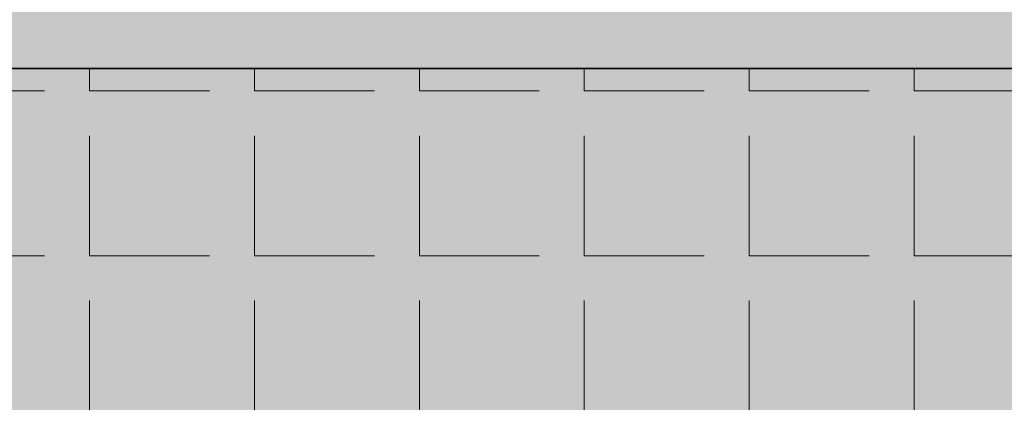
# Model space of a CAD drawing. Units: millimetres. Extents: x 1166 to 16630, y -7192 to 2820.
# Tile 4 of 8: x 5842 to 7051, y -3052 to -2583. Entities that reach past the tile are written whole.
import ezdxf

# ---------------------------------------------------------------- set-up
doc = ezdxf.new("R2010")
doc.units = ezdxf.units.MM
doc.layers.add('A-FLOR-FNSH-PATT', color=254, linetype='Continuous', lineweight=13, true_color=0xfeeab9)
doc.layers.add('A-WALL-PATT', color=254, linetype='Continuous', lineweight=13, true_color=0xcecce6)
doc.layers.add('A-FLOR-PATT', color=8, linetype='Continuous', lineweight=13)
doc.layers.add('A-WALL', color=7, linetype='Continuous', lineweight=35)

msp = doc.modelspace()

# ---------------------------------------------------------------- hatches: boundary and pattern name
at = {"layer": 'A-FLOR-FNSH-PATT', "transparency": 33554523}
h = msp.add_hatch(color=256, dxfattribs=at)
h.dxf.hatch_style = 1
h.paths.add_polyline_path([(7725.939441137629, 2327.46223509218), (1725.939441137629, 2327.46223509218), (1725.939441137629, -5672.537764907821), (5309.614992693758, -5672.537764907821), (5309.614992693758, -2642.53776490782), (5189.614992693758, -2642.53776490782), (5189.614992693758, -5442.537764907821), (1955.939441137629, -5442.537764907819), (1955.939441137628, 2097.46223509218), (4665.939441137629, 2097.46223509218), (4665.939441137629, 150.2003357952274), (4815.939441137629, 150.2003357952271, -0.4014527144963571), (5814.98195149442, -806.0496642047723), (5815.939441137629, -806.0496642047722), (5815.939441137629, -849.7996642047723), (4815.939441137629, -849.7996642047729), (4785.939441137628, -849.7996642047729), (4785.939441137628, -902.5377649078198), (7495.939441137629, -902.5377649078199), (7495.939441137629, -2522.53776490782), (4884.014389835691, -2522.53776490782), (4884.014389835691, -2642.53776490782), (7725.939441137629, -2642.53776490782)], flags=17)
h.paths.add_polyline_path([(6066.077252941604, 618.4211469541298), (6066.077252941604, 1624.186122025141), (7407.097946088891, 1624.186122025141), (7407.097946088891, 618.4211469541295)], flags=16)
h.paths.add_polyline_path([(4979.211803565785, 660.218557639132), (4799.278299447288, 660.218557639132), (4799.278299447288, 780.1742270514636), (4789.281993662927, 790.1705328358245), (4789.281993662927, 870.1409791107119), (4799.278299447288, 880.137284895073), (4799.278299447288, 1259.996904700789), (4979.211803565785, 1259.996904700789), (4979.211803565785, 1230.007987347706), (4989.208109350147, 1230.007987347706), (4989.208109350147, 1110.052317935374), (4979.211803565785, 1110.052317935374), (4979.211803565785, 1100.056012151014), (4989.208109350147, 1100.056012151014), (4989.208109350147, 980.1003427386823), (4979.211803565785, 980.1003427386823), (4979.211803565785, 950.1114253855995), (4989.208109350147, 950.1114253855995), (4989.208109350147, 940.1151196014531, -0.0909090909092653), (4989.208109350147, 720.1963923450827), (4989.208109350147, 710.2000865609368), (4979.211803565785, 710.2000865609368)], flags=16)
h.paths.add_polyline_path([(4974.213650673605, 665.2167105313125), (4804.276452339468, 665.2167105313125), (4804.276452339468, 1254.998751808608), (4974.213650673605, 1254.998751808608)], flags=0)
h.paths.add_polyline_path([(6910.920475690947, 618.4211469541297), (6910.920475690947, 873.2148154769015), (7165.714311841242, 873.2148154769015), (7165.714311841242, 1490.084270626194), (7386.982643234919, 1490.084270626193), (7386.982643234919, 1141.419188784891), (7165.714311841242, 1141.419188784891), (7165.714311841242, 1101.188415449426), (7386.98264323492, 1101.188415449426), (7386.98264323492, 752.5231659806007), (7132.188807084624, 752.5231659806008), (7132.188807084624, 839.6893327765368)], flags=16)
h.paths.add_polyline_path([(4815.93944113763, 150.200335795227), (4665.939441137629, 150.2003357952274), (4665.939441137629, 1500.696746688973), (2460.544987272565, 1500.696746688973), (2460.544987272566, -402.5377649078198), (3575.939441137629, -402.5377649078199), (3575.93944113763, -1706.640093510054), (3463.439441137629, -1706.640093510054, 0.4014527144963571), (2714.157558370035, -2423.827593510054), (3463.439441137629, -2423.827593510054), (3463.439441137629, -2456.640093510054), (3455.939441137629, -2522.53776490782), (3455.939441137628, -2456.640093510053), (2713.439441137629, -2456.640093510054), (2713.439441137629, -2423.827593510054), (2714.157558370035, -2423.827593510054, -0.398552660000795), (3455.939441137629, -1706.6775944476), (3455.93944113763, -1706.640093510053), (3575.939441137629, -1706.640093510054), (3575.939441137629, -402.5377649078199), (2460.544987272566, -402.5377649078199), (2460.544987272565, 1500.696746688973), (4665.939441137629, 1500.696746688972), (4665.939441137629, 150.2003357952274), (4785.939441137628, 150.2003357952272), (4785.939441137628, 2097.46223509218), (7495.939441137629, 2097.46223509218), (7495.939441137629, -2522.53776490782), (4884.014389835691, -2522.53776490782), (4884.014389835691, -2642.53776490782), (7725.939441137629, -2642.53776490782), (7725.939441137629, 2327.46223509218), (1725.939441137629, 2327.46223509218), (1725.939441137629, -5672.537764907822), (5309.614992693758, -5672.53776490782), (5309.614992693758, -2642.53776490782), (4884.014389835691, -2642.53776490782), (4884.014389835691, -2522.53776490782), (4884.014389835691, -1822.53776490782), (4665.939441137629, -1822.53776490782), (4665.939441137629, -1722.53776490782), (4665.939441137629, -1022.53776490782), (4665.939441137629, -849.7996642047729), (4815.939441137629, -849.7996642047725), (4815.939441137629, -806.0496642047731), (5814.98195149442, -806.0496642047723, 0.4014527144963566)])
h.paths.add_polyline_path([(1955.939441137629, -4323.626378184433), (1965.93574692199, -4313.63007240007), (1965.93574692199, -3933.770452594356), (2145.869251040488, -3933.770452594356), (2145.869251040488, -3963.759369947439), (2155.865556824849, -3963.759369947439), (2155.865556824849, -4083.715039359769), (2145.869251040488, -4083.715039359769), (2145.869251040488, -4093.711345144131), (2155.865556824848, -4093.711345144131), (2155.865556824848, -4213.667014556462), (2145.869251040487, -4213.667014556462), (2145.869251040487, -4243.655931909545), (2155.865556824848, -4243.655931909545), (2155.865556824848, -4253.65223769369, -0.0909090909092649), (2155.865556824848, -4473.570964950059), (2155.865556824849, -4483.567270734208), (2145.869251040488, -4483.567270734208), (2145.869251040487, -4533.548799656013), (1965.935746921989, -4533.548799656013), (1965.93574692199, -4413.593130243681), (1955.939441137628, -4403.596824459319)], flags=16)
h.paths.add_polyline_path([(3017.671753088376, -1268.685150923248), (3017.671753088376, -1558.932187923503), (2092.537854326397, -1558.932187923502), (2092.537854326398, -1268.685150923248)], flags=16)
h.paths.add_polyline_path([(2768.798554444471, -687.0284595558132), (2664.903705041528, -687.0284595558132), (2696.87076529663, -782.9296403211201, -0.5013234908366285), (2617.666699633876, -1084.404517764256, -0.1328909081875925), (2584.270795046388, -1084.404517500901, -0.5013167773011727), (2505.0649162136, -782.9330743979611), (2537.033121160982, -687.0284595558132), (2489.081652205777, -687.028459555813), (2489.081652205777, -711.0041940334156), (2441.130183250573, -711.0041940334156), (2441.130183250573, -687.0284595558132), (2433.138271758039, -687.0284595558132), (2433.138271758038, -559.1578756752677), (2768.79855444447, -559.1578756752677)], flags=16)
h.paths.add_polyline_path([(2752.814731459403, -655.0608109277462, -0.4142135623730841), (2740.826866878533, -671.0446365707452), (2465.105920386106, -671.0446365707452, -0.4142135623731292), (2449.122094743107, -659.056771989874), (2449.122094743107, -591.1255243033348, -0.414213562373052), (2461.109959323975, -575.141698660336), (2736.830905816402, -575.141698660336, -0.4142135623731314), (2752.814731459403, -587.1295632412064)], flags=0)
h.paths.add_polyline_path([(2627.246667254749, -1063.015793855159, -0.2150037826741433), (2574.690827957569, -1063.015793301976, -0.4800796505542296), (2537.033991046724, -782.9313974662225), (2664.904416594217, -782.9313974662225, -0.4800795019661017)], flags=0)
h.paths.add_polyline_path([(4505.633741405676, -3647.875139181167), (4977.86337820884, -3647.875139181167, -0.190476207544349), (4977.863715650206, -5173.540873043219), (4505.633741405676, -5173.540873043219), (4505.633741405676, -5064.564758277272), (4533.929389604653, -5064.564758277272), (4533.929389604654, -3756.851253947113), (4505.633741405676, -3756.851253947113)], flags=16)
h.paths.add_polyline_path([(4880.113813381636, -4192.755706203317), (5003.372332977528, -4192.75565851188, -0.0496282101666582), (5003.372387193955, -4628.660299224469), (4880.113813381636, -4628.660251533011)], flags=0)
h.paths.add_polyline_path([(2140.871098148307, -3938.768605486535), (2140.871098148307, -4528.550646763831), (1970.933899814171, -4528.550646763831), (1970.93389981417, -3938.768605486536)], flags=0)
h.paths.add_polyline_path([(7495.939441137629, -1022.53776490782), (6660.698736718376, -1022.53776490782), (6660.698736718376, -1722.53776490782, -0.2129119084378026), (6697.901439354037, -1739.131793636166)], flags=16)
h.paths.add_polyline_path([(7495.939441137629, -1022.53776490782), (6697.901439354037, -1739.131793636166, -0.1849874276879184), (6710.698736718376, -1772.53776490782), (7495.939441137629, -1772.53776490782)], flags=16)
h.paths.add_polyline_path([(7495.939441137629, -1772.53776490782), (6710.698736718376, -1772.53776490782, -0.1849874276879184), (6697.901439354037, -1805.943736179474), (7495.939441137629, -2522.53776490782)], flags=16)
h.paths.add_polyline_path([(6697.901439354037, -1805.943736179474, -0.2129119084378014), (6660.698736718376, -1822.53776490782), (6660.698736718376, -2522.53776490782), (7495.939441137629, -2522.53776490782)], flags=16)
h.paths.add_polyline_path([(6660.698736718376, -1822.53776490782), (6438.61319335804, -1822.53776490782), (6438.61319335804, -2522.53776490782), (6660.698736718376, -2522.53776490782)], flags=16)
h.paths.add_polyline_path([(6438.61319335804, -1822.53776490782), (6216.527649997704, -1822.53776490782), (6216.527649997704, -2522.53776490782), (6438.61319335804, -2522.53776490782)], flags=16)
h.paths.add_polyline_path([(6216.527649997704, -1822.53776490782), (5994.442106637368, -1822.53776490782), (5994.442106637369, -2522.53776490782), (6216.527649997704, -2522.53776490782)], flags=16)
h.paths.add_polyline_path([(5994.442106637368, -1822.53776490782), (5772.356563277032, -1822.53776490782), (5772.356563277033, -2522.53776490782), (5994.442106637369, -2522.53776490782)], flags=16)
h.paths.add_polyline_path([(5550.271019916698, -1822.53776490782), (5328.185476556361, -1822.53776490782), (5328.185476556362, -2522.53776490782), (5550.271019916698, -2522.53776490782)], flags=16)
h.paths.add_polyline_path([(5328.185476556361, -1822.53776490782), (5106.099933196027, -1822.53776490782), (5106.099933196027, -2522.53776490782), (5328.185476556362, -2522.53776490782)], flags=16)
h.paths.add_polyline_path([(5106.099933196027, -1822.53776490782), (4884.014389835691, -1822.53776490782), (4884.014389835691, -2522.53776490782), (5106.099933196027, -2522.53776490782)], flags=16)
h.paths.add_polyline_path([(4884.014389835691, -1022.53776490782), (4665.939441137629, -1022.53776490782), (4665.939441137629, -1722.53776490782), (4884.014389835691, -1722.53776490782)], flags=16)
h.paths.add_polyline_path([(5106.099933196027, -1022.53776490782), (4884.014389835691, -1022.53776490782), (4884.014389835691, -1722.53776490782), (5106.099933196027, -1722.53776490782)], flags=16)
h.paths.add_polyline_path([(5550.271019916698, -1022.53776490782), (5328.185476556362, -1022.53776490782), (5328.185476556361, -1722.53776490782), (5550.271019916698, -1722.53776490782)], flags=16)
h.paths.add_polyline_path([(5328.185476556362, -1022.53776490782), (5106.099933196027, -1022.53776490782), (5106.099933196027, -1722.53776490782), (5328.185476556361, -1722.53776490782)], flags=16)
h.paths.add_polyline_path([(5772.356563277033, -1022.53776490782), (5550.271019916698, -1022.53776490782), (5550.271019916698, -1722.53776490782), (5772.356563277032, -1722.53776490782)], flags=16)
h.paths.add_polyline_path([(5994.442106637369, -1022.53776490782), (5772.356563277033, -1022.53776490782), (5772.356563277032, -1722.53776490782), (5994.442106637368, -1722.53776490782)], flags=16)
h.paths.add_polyline_path([(6216.527649997704, -1022.53776490782), (5994.442106637369, -1022.53776490782), (5994.442106637368, -1722.53776490782), (6216.527649997704, -1722.53776490782)], flags=16)
h.paths.add_polyline_path([(6660.698736718376, -1022.53776490782), (6438.61319335804, -1022.53776490782), (6438.61319335804, -1722.53776490782), (6660.698736718376, -1722.53776490782)], flags=16)
h.paths.add_polyline_path([(6438.61319335804, -1022.53776490782), (6216.527649997704, -1022.53776490782), (6216.527649997704, -1722.53776490782), (6438.61319335804, -1722.53776490782)], flags=16)
h.paths.add_polyline_path([(5772.356563277032, -1822.53776490782), (5550.271019916698, -1822.53776490782), (5550.271019916698, -2522.53776490782), (5772.356563277033, -2522.53776490782)], flags=16)
h.paths.add_polyline_path([(6660.698736718376, -1722.53776490782), (6438.61319335804, -1722.53776490782), (4665.939441137629, -1722.537764907819), (4665.939441137629, -1822.53776490782), (6660.698736718376, -1822.53776490782, 0.2129119084377995), (6697.901439354037, -1805.943736179474, 0.6489243663012206)], flags=16)
h.paths.add_polyline_path([(5860.250212969285, -44.00639852248207), (7154.50411478644, -44.00639852248207), (7154.50411478644, 215.6889194604054), (5860.250212969285, 215.6889194604054)], flags=24)
h.paths.add_polyline_path([(2102.335631979146, -1543.656328414819), (3007.075088498303, -1543.656328414819), (3007.075088498303, -1283.961010431932), (2102.335631979146, -1283.961010431932)], flags=8)
h.paths.add_polyline_path([(2887.503040984853, -4248.680096729577), (3740.371909930631, -4248.680096729577), (3740.371909930631, -3989.155968804687), (2887.503040984853, -3989.155968804687)], flags=24)
h.paths.add_polyline_path([(2999.435985189627, 433.0535291407016), (4111.828982060295, 433.0535291407016), (4111.828982060295, 692.5776570655913), (2999.435985189627, 692.5776570655913)], flags=24)
at = {"layer": 'A-FLOR-FNSH-PATT', "transparency": 33554590}
h = msp.add_hatch(color=256, dxfattribs=at)
h.dxf.hatch_style = 1
h.paths.add_polyline_path([(5309.614992693758, -2642.53776490782), (5309.614992693758, -6304.141088113749), (7725.939441137629, -6304.141088113749), (7725.939441137629, -5672.53776490782), (7725.939441137629, -2642.53776490782)])
edge = h.paths.add_edge_path(flags=16)
edge.add_ellipse((-448.9724108440159, -3645.429588524165), major_axis=(-7430.722679011307, 2.05049e-10), ratio=0.8423038695440578, start_angle=182.1799503136468, end_angle=183.6504275857006, ccw=False)
edge.add_line((6974.17381326888, -3362.862478220109), (6984.715647929133, -3362.862478220109))
edge.add_ellipse((6982.28108362224, -3380.396843230207), major_axis=(-20.81714882728829, 5.19e-13), ratio=0.842303869543992, start_angle=180.0000000000014, end_angle=270.0000000000014, ccw=False)
edge.add_line((7003.098232449528, -3380.396843230198), (7003.098232449528, -3722.915565549822))
edge.add_ellipse((6982.28108362224, -3720.864922613471), major_axis=(20.81714882728829, 5.097e-13), ratio=0.842303869543992, start_angle=269.9999999999985, end_angle=359.9999999999986, ccw=False)
edge.add_ellipse((-142030.922985108, -3973.064272051784), major_axis=(149013.2040687302, 7.3876543e-09), ratio=0.8423038695454406, start_angle=-0.3838667787953227, end_angle=0.09022908859151357, ccw=False)
edge.add_line((6977.567346638728, -4971.397229994678), (6984.470063297348, -4971.397229994678))
edge.add_ellipse((6982.28108362224, -4988.931595004776), major_axis=(20.81714882728829, 5.4695e-12), ratio=0.84230386954397, start_angle=-1.5006662579253316e-11, end_angle=89.99999999998488, ccw=False)
edge.add_line((7003.098232449528, -4988.931595004766), (7003.098232449527, -5331.243460438734))
edge.add_ellipse((6982.281083622239, -5329.399674388036), major_axis=(-20.81714882728829, 1.0505e-12), ratio=0.84230386954397, start_angle=90.0000000000029, end_angle=180.000000000003, ccw=False)
edge.add_line((6982.281083622243, -5346.934039398132), (6973.353954790083, -5346.934039398132))
edge.add_ellipse((-142030.922985108, -3973.064272051784), major_axis=(149013.2040687302, 7.3876543e-09), ratio=0.8423038695454406, start_angle=-0.6186431963221253, end_angle=-0.5282714718208013, ccw=False)
edge.add_ellipse((6960.189207408767, -5606.902802775503), major_axis=(-31.22572324093233, 2.0889e-12), ratio=0.8423038695439425, start_angle=179.3717627838109, end_angle=248.4647566010108, ccw=False)
edge.add_ellipse((-142041.331559525, -3973.064272085929), major_axis=(-149045.3717863939, 4.64621177404e-05), ratio=0.8423038661083152, start_angle=179.3534459208122, end_angle=179.3717628016453, ccw=False)
edge.add_ellipse((6916.869834512962, -5654.054118847628), major_axis=(-73.80201542105252, 3.6097e-12), ratio=0.8423038695439748, start_angle=90.00000000006492, end_angle=179.353445902922, ccw=False)
edge.add_line((6916.869834513031, -5716.217842016925), (5995.230132669023, -5716.217842016909))
edge.add_ellipse((5995.230132669163, -5654.054118847574), major_axis=(73.80201542109666, 3.978e-13), ratio=0.8423038695439887, start_angle=180.6465540970575, end_angle=269.9999999998622, ccw=False)
edge.add_ellipse((154953.4315273228, -3973.06427200764), major_axis=(-149045.3717871212, 2.2898328512e-06), ratio=0.8423038697262194, start_angle=0.6282372171232851, end_angle=0.6465540979564253, ccw=False)
edge.add_ellipse((5951.910759773294, -5606.902802775455), major_axis=(31.22572324094488, 4.9039e-12), ratio=0.842303869543988, start_angle=111.53524350401449, end_angle=180.6282372161637, ccw=False)
edge.add_ellipse((154943.0229527065, -3973.064272049507), major_axis=(-149013.2040691466, 7.4869171e-09), ratio=0.8423038695459824, start_angle=0.528271471820176, end_angle=0.6465540970638131, ccw=False)
edge.add_line((5938.746012391977, -5346.934039398132), (5927.384319252956, -5346.934039398132))
edge.add_ellipse((5929.818883559845, -5329.399674388033), major_axis=(20.8171488272892, 3.11e-13), ratio=0.8423038695440205, start_angle=179.9999999999992, end_angle=269.9999999999962, ccw=False)
edge.add_line((5909.001734732555, -5329.399674388034), (5909.001734732554, -4986.88095206843))
edge.add_ellipse((5929.818883559843, -4988.931595004776), major_axis=(-20.8171488272892, 3.063e-13), ratio=0.8423038695440205, start_angle=-89.99999999999608, end_angle=7.958078640513122e-13, ccw=False)
edge.add_line((5929.818883559843, -4971.397229994676), (5934.53262054336, -4971.397229994676))
edge.add_ellipse((154943.0229527065, -3973.064272049507), major_axis=(-149013.2040691466, 7.4869171e-09), ratio=0.8423038695459824, start_angle=-0.09022908859031986, end_angle=0.38386677879520903, ccw=False)
edge.add_ellipse((5929.818883559843, -3720.864922613471), major_axis=(-20.8171488272892, 1.5867e-12), ratio=0.8423038695439331, start_angle=4.376943252282217e-12, end_angle=90.00000000000438, ccw=False)
edge.add_line((5909.001734732555, -3720.864922613478), (5909.001734732555, -3378.346200293855))
edge.add_ellipse((5929.818883559843, -3380.396843230207), major_axis=(20.8171488272892, 9.396e-13), ratio=0.8423038695439548, start_angle=89.99999999999739, end_angle=179.9999999999975, ccw=False)
edge.add_line((5929.818883559843, -3362.862478220109), (5937.926153913206, -3362.862478220109))
edge.add_ellipse((13361.0723780261, -3645.42958852417), major_axis=(7430.722679011307, 7.96527e-11), ratio=0.8423038695440075, start_angle=176.3495724143003, end_angle=177.8200496863542, ccw=False)
edge.add_ellipse((6843.238962592569, -6808.26137511002), major_axis=(4407.332901654202, 4.993684e-10), ratio=0.8423038695438785, start_angle=102.12596555227748, end_angle=103.7805289894913, ccw=False)
edge.add_ellipse((6843.238962592481, -6711.831352601092), major_axis=(4294.727564406183, 8.108409e-10), ratio=0.8423038695438188, start_angle=100.20953899713243, end_angle=102.4446272934332, ccw=False)
edge.add_ellipse((5718.978043047074, -189.3416182050969), major_axis=(-3530.283493235897, 2.29487e-11), ratio=0.8423038695439934, start_angle=99.25656600720184, end_angle=102.5549326441376)
edge.add_line((6369.842688727707, -3111.939026631001), (6452.046781461999, -3066.482546539763))
edge.add_ellipse((6456.049983591043, -3074.756545497792), major_axis=(-10.40857441364578, 1.5838e-12), ratio=0.8423038695437935, start_angle=270.0000000000206, end_angle=307.9331304598557, ccw=False)
edge.add_ellipse((6456.049983591043, -3074.756545497792), major_axis=(-10.40857441364578, 1.5838e-12), ratio=0.8423038695437935, start_angle=232.06686954016618, end_angle=270.0000000000206, ccw=False)
edge.add_line((6461.762224667734, -3067.427595530816), (6542.257278454378, -3111.939026631002))
edge.add_ellipse((7193.121924135012, -189.3416182050969), major_axis=(3530.283493235459, 5.426614e-10), ratio=0.842303869544094, start_angle=257.4450673558539, end_angle=260.7434339927895)
edge.add_ellipse((6068.861004589511, -6711.831352601148), major_axis=(4294.72756440461, 7.517164e-10), ratio=0.8423038695441345, start_angle=77.55537270654469, end_angle=79.79046100284552, ccw=False)
edge.add_ellipse((6068.86100458951, -6808.26137511002), major_axis=(-4407.332901654327, 6.637773e-10), ratio=0.842303869543856, start_angle=256.2194710105107, end_angle=257.8740344477245, ccw=False)
edge = h.paths.add_edge_path(flags=0)
edge.add_ellipse((5799.636342679871, -3484.80630294614), major_axis=(790.1331889300527, 2.1537e-12), ratio=0.8423038695439757, start_angle=-2.2737367544323206e-13, end_angle=29.43856959797921, ccw=False)
edge.add_line((6589.769531609924, -3484.806302946152), (6589.769531609924, -3517.865771969153))
edge.add_line((6589.769531609924, -3517.865771969153), (6615.396946753699, -3517.865771969153))
edge.add_ellipse((6612.950235160742, -3526.632954474201), major_axis=(10.40857441364348, 1.5653e-12), ratio=0.8423038695440233, start_angle=45.51978911742219, end_angle=89.99999999999147, ccw=False)
edge.add_line((6619.58436781158, -3519.877346340421), (6697.576744801804, -3574.216072032502))
edge.add_line((6697.576744801804, -3574.216072032502), (6697.576744801804, -3782.552340767745))
edge.add_ellipse((6643.673138205864, -3780.461483581003), major_axis=(5.016450041930374, 89.18653102701357), ratio=0.6038335755719256, start_angle=106.34259195429391, end_angle=270.99798572497, ccw=False)
edge.add_line((6589.769531609924, -3793.028339937766), (6589.769531609924, -3484.806302946153))
edge.add_ellipse((5799.636342679871, -3484.80630294614), major_axis=(790.1331889300527, 2.1537e-12), ratio=0.8423038695439757, start_angle=-2.143e-13, end_angle=29.43856959797918)
edge.add_ellipse((7112.463624502211, -3484.80630294614), major_axis=(-790.1331889300524, 7.9434e-12), ratio=0.8423038695439707, start_angle=-29.43856959797882, end_angle=5.465e-13)
edge.add_line((6322.330435572158, -3484.806302946151), (6322.330435572158, -3793.028339937766))
edge.add_ellipse((6268.426828976219, -3780.461483581003), major_axis=(-5.016450041930374, 89.18653102701357), ratio=0.6038335755719256, start_angle=89.00201427502998, end_angle=253.6574080457062, ccw=False)
edge.add_line((6214.523222380278, -3782.552340767737), (6214.523222380279, -3574.216072032502))
edge.add_line((6214.523222380279, -3574.216072032502), (6294.400928520307, -3518.563802793423))
edge.add_ellipse((6299.149732021341, -3526.632954474201), major_axis=(10.4085744136453, 3.381e-13), ratio=0.8423038695438764, start_angle=89.9999999999983, end_angle=134.4802108825654, ccw=False)
edge.add_line((6299.149732021338, -3517.865771969152), (6322.330435572158, -3517.865771969152))
edge.add_line((6322.330435572158, -3517.865771969152), (6322.330435572158, -3484.806302946154))
edge.add_ellipse((7112.463624502211, -3484.80630294614), major_axis=(-790.1331889300524, 7.9434e-12), ratio=0.8423038695439707, start_angle=-29.438569597978812, end_angle=6.252776074688882e-13, ccw=False)
edge = h.paths.add_edge_path(flags=0)
edge.add_line((6899.672020630411, -4051.112638739672), (6868.937058315451, -4281.473694083312))
edge.add_ellipse((6495.430033257824, -5170.362894493258), major_axis=(1119.455420763322, 3.0514e-12), ratio=0.8423038695439744, start_angle=67.20808512240981, end_angle=85.12993040286408)
edge.add_line((6575.564661792019, -4229.860228440724), (6336.53530539007, -4229.860228440724))
edge.add_ellipse((6416.669933924288, -5170.362894493482), major_axis=(1119.455420763633, 5.82337e-11), ratio=0.842303869543943, start_angle=94.87006959713275, end_angle=112.7919148775836)
edge.add_line((6043.162908866626, -4281.473694083309), (6012.427946551666, -4051.112638739666))
edge.add_ellipse((6380.264280565288, -4969.144446445703), major_axis=(1150.303461305961, 5.9583e-11), ratio=0.8423038695439412, start_angle=94.27742096305099, end_angle=111.83495379670521, ccw=False)
edge.add_line((6307.939299228742, -4002.156437400477), (6604.160667953341, -4002.156437400477))
edge.add_ellipse((6531.835686616772, -4969.144446445682), major_axis=(-1150.303461305901, 2.25473e-11), ratio=0.8423038695439672, start_angle=248.1650462032914, end_angle=265.72257903694555, ccw=False)
edge = h.paths.add_edge_path(flags=0)
edge.add_ellipse((-142030.9229855244, -3973.064272050007), major_axis=(-148992.3869203194, 2.076209e-10), ratio=0.842303869544003, start_angle=179.6222358060902, end_angle=179.9444056865007, ccw=False)
edge.add_line((6956.899516505626, -4955.389335168179), (6903.06848209712, -4744.029778632651))
edge.add_ellipse((-45118.92430422086, -4413.460367112857), major_axis=(52023.47313689829, 7.771381e-10), ratio=0.842303869543516, start_angle=-0.3640763488911976, end_angle=0.1208973690317991)
edge.add_line((6904.3855953652, -4303.688047353878), (6961.365076797346, -4117.63210307358))
edge = h.paths.add_edge_path(flags=0)
edge.add_line((5950.734890384741, -4117.632103073563), (6007.714371816899, -4303.688047353918))
edge.add_ellipse((58031.02427140294, -4413.460367113082), major_axis=(-52023.47313689826, 1.3200601e-09), ratio=0.8423038695497072, start_angle=-0.1208973690315197, end_angle=0.364076348891516)
edge.add_line((6009.031485084967, -4744.029778632643), (5955.200450676423, -4955.389335168309))
edge.add_ellipse((154943.0229527063, -3973.064272050686), major_axis=(-148992.3869203192, 3.28274152e-08), ratio=0.8423038695536886, start_angle=0.05559431351167632, end_angle=0.3777641939223031, ccw=False)
edge = h.paths.add_edge_path(flags=0)
edge.add_line((6868.937058315452, -5013.198477251068), (6868.937058315452, -5277.993200767081))
edge.add_ellipse((6456.049983591043, -3571.079447459644), major_axis=(2068.11644385622, 7.9333e-12), ratio=0.8423038695439821, start_angle=256.4018653097692, end_angle=283.59813469023027, ccw=False)
edge.add_line((6043.16290886663, -5277.993200767081), (6043.16290886663, -5013.198477251068))
edge.add_ellipse((6456.049983591043, -3306.284723943631), major_axis=(2068.116443856253, 3.3411e-12), ratio=0.8423038695439679, start_angle=256.4018653097692, end_angle=283.5981346902304)
edge = h.paths.add_edge_path(flags=0)
edge.add_ellipse((6827.302760660877, -5415.313265203762), major_axis=(-41.63429765457658, 1.038e-12), ratio=0.842303869543992, start_angle=180.0000000000014, end_angle=270.0000000000014, ccw=False)
edge.add_line((6868.937058315454, -5415.313265203762), (6868.937058315454, -5689.12284886784))
edge.add_line((6868.937058315454, -5689.12284886784), (6043.162908866631, -5689.122848867824))
edge.add_line((6043.162908866631, -5689.122848867824), (6043.16290886663, -5415.313265203758))
edge.add_ellipse((6084.797206521206, -5415.313265203759), major_axis=(-41.63429765457658, 3.4138e-12), ratio=0.842303869543992, start_angle=-89.99999999999523, end_angle=4.718003765447065e-12, ccw=False)
edge.add_line((6084.797206521207, -5380.244535183563), (6827.302760660879, -5380.244535183566))
h.paths.add_polyline_path([(3455.939441137629, -522.53776490782), (1955.939441137629, -522.53776490782), (1955.939441137629, -2522.53776490782), (3455.939441137629, -2522.53776490782), (3455.939441137628, -2456.640093510054), (2713.439441137629, -2456.640093510054), (2713.43944113763, -2423.827593510054), (2714.157558370035, -2423.827593510054, -0.398552660000795), (3455.939441137629, -1706.6775944476)])
h.paths.add_polyline_path([(2617.666699633915, -1084.404517764245, -0.1328909081885223), (2584.2707950462, -1084.404517500826, -0.5013167773008519), (2505.064916213601, -782.9330743979599), (2537.033121160981, -687.0284595558127), (2489.081652205778, -687.0284595558132), (2489.081652205778, -711.0041940334158), (2441.130183250573, -711.0041940334158), (2441.130183250573, -695.0203710483474), (2473.097829220709, -695.0203710483474), (2473.097829220709, -687.0284595558132), (2433.13827175804, -687.0284595558132), (2433.138271758038, -559.1578756752674), (2768.79855444447, -559.1578756752674), (2768.798554444471, -687.0284595558132), (2664.903705041528, -687.0284595558132), (2696.870765296628, -782.9296403211174, -0.5013234908365807)], flags=16)
h.paths.add_polyline_path([(2627.246667254758, -1063.015793855155, -0.2150037826753064), (2574.690827957319, -1063.015793301825, -0.4800796505537303), (2537.033991046725, -782.9313974662227), (2664.904416594217, -782.9313974662227, -0.4800795019660876)], flags=0)
h.paths.add_polyline_path([(2736.830905816404, -671.0446365707452), (2465.105920386107, -671.0446365707452, -0.5000001164022092), (2449.122094743107, -655.0608109277463), (2449.122094743107, -591.1255243033341, -0.5000001164022404), (2465.105920386111, -575.1416986603361), (2736.830905816402, -575.1416986603361, -0.5000001164023353), (2752.814731459403, -591.1255243033406), (2752.814731459403, -655.0608109277468, -0.50000011640211)], flags=0)
h.paths.add_polyline_path([(5931.781743219382, -6111.826019846759), (7070.309755611069, -6111.826019846759), (7070.309755611069, -5852.301891921869), (5931.781743219382, -5852.301891921869)], flags=24)
h.paths.add_polyline_path([(2102.335631979146, -1543.656328414819), (3007.075088498303, -1543.656328414819), (3007.075088498303, -1283.961010431932), (2102.335631979146, -1283.961010431932)], flags=24)
at = {"layer": 'A-FLOR-PATT', "transparency": 33554564}
h = msp.add_hatch(dxfattribs=at)
h.set_pattern_fill('ANGLE', color=256, scale=29)
h.set_pattern_definition([(0, (-8657.519420588213, -11987.85165359825), (0, 202.565), [147.32, -55.24499999999999]), (90, (-8657.519420588213, -11987.85165359825), (-202.565, 1.24e-14), [147.32, -55.24499999999999])])
h.paths.add_polyline_path([(7725.939441137629, -2642.53776490782), (5309.614992693758, -2642.53776490782), (5309.614992693758, -6304.141088113749), (7725.939441137629, -6304.141088113749), (7725.939441137629, -5672.53776490782)])
edge = h.paths.add_edge_path(flags=16)
edge.add_ellipse((-142030.922985108, -3973.064272051784), major_axis=(149013.2040687302, 7.3876543e-09), ratio=0.8423038695454406, start_angle=-0.3838667787953227, end_angle=0.09022908859151357, ccw=False)
edge.add_ellipse((6982.28108362224, -4988.931595004776), major_axis=(20.81714882728829, 5.4695e-12), ratio=0.84230386954397, start_angle=-1.5006662579253316e-11, end_angle=89.99999999998488, ccw=False)
edge.add_line((7003.098232449528, -4988.931595004773), (7003.098232449527, -5329.399674388036))
edge.add_ellipse((6982.281083622239, -5329.399674388036), major_axis=(-20.81714882728829, 1.0505e-12), ratio=0.84230386954397, start_angle=90.0000000000029, end_angle=180.000000000003, ccw=False)
edge.add_line((6982.281083622241, -5346.934039398132), (6973.353954790083, -5346.934039398132))
edge.add_ellipse((-142030.922985108, -3973.064272051784), major_axis=(149013.2040687302, 7.3876543e-09), ratio=0.8423038695454406, start_angle=-0.6186431963221253, end_angle=-0.5282714718208013, ccw=False)
edge.add_ellipse((6960.189207408767, -5606.902802775503), major_axis=(-31.22572324093233, 2.0889e-12), ratio=0.8423038695439425, start_angle=179.3717627838109, end_angle=248.4647566010108, ccw=False)
edge.add_ellipse((-142041.331559525, -3973.064272085929), major_axis=(-149045.3717863939, 4.64621177404e-05), ratio=0.8423038661083152, start_angle=179.3534459208122, end_angle=179.3717628016453, ccw=False)
edge.add_ellipse((6916.869834512962, -5654.054118847628), major_axis=(-73.80201542105252, 3.6097e-12), ratio=0.8423038695439748, start_angle=90.00000000006492, end_angle=179.353445902922, ccw=False)
edge.add_line((6916.869834513029, -5716.217842016925), (5995.230132669016, -5716.217842016909))
edge.add_ellipse((5995.230132669163, -5654.054118847574), major_axis=(73.80201542109666, 3.978e-13), ratio=0.8423038695439887, start_angle=180.6465540970575, end_angle=269.9999999998622, ccw=False)
edge.add_ellipse((154953.4315273228, -3973.06427200764), major_axis=(-149045.3717871212, 2.2898328512e-06), ratio=0.8423038697262194, start_angle=0.6282372171232851, end_angle=0.6465540979564253, ccw=False)
edge.add_ellipse((5951.910759773294, -5606.902802775455), major_axis=(31.22572324094488, 4.9039e-12), ratio=0.842303869543988, start_angle=111.53524350401449, end_angle=180.6282372161637, ccw=False)
edge.add_ellipse((154943.0229527065, -3973.064272049507), major_axis=(-149013.2040691466, 7.4869171e-09), ratio=0.8423038695459824, start_angle=0.528271471820176, end_angle=0.6465540970638131, ccw=False)
edge.add_line((5938.746012391977, -5346.934039398132), (5929.818883559843, -5346.934039398132))
edge.add_ellipse((5929.818883559845, -5329.399674388033), major_axis=(20.8171488272892, 3.11e-13), ratio=0.8423038695440205, start_angle=179.9999999999992, end_angle=269.9999999999962, ccw=False)
edge.add_line((5909.001734732555, -5329.399674388033), (5909.001734732554, -4988.931595004778))
edge.add_ellipse((5929.818883559843, -4988.931595004776), major_axis=(-20.8171488272892, 3.063e-13), ratio=0.8423038695440205, start_angle=-89.99999999999608, end_angle=7.958078640513122e-13, ccw=False)
edge.add_ellipse((154943.0229527065, -3973.064272049507), major_axis=(-149013.2040691466, 7.4869171e-09), ratio=0.8423038695459824, start_angle=-0.09022908859031986, end_angle=0.38386677879520903, ccw=False)
edge.add_ellipse((5929.818883559843, -3720.864922613471), major_axis=(-20.8171488272892, 1.5867e-12), ratio=0.8423038695439331, start_angle=4.376943252282217e-12, end_angle=90.00000000000438, ccw=False)
edge.add_line((5909.001734732555, -3720.864922613472), (5909.001734732555, -3380.396843230204))
edge.add_ellipse((5929.818883559843, -3380.396843230207), major_axis=(20.8171488272892, 9.396e-13), ratio=0.8423038695439548, start_angle=89.99999999999739, end_angle=179.9999999999975, ccw=False)
edge.add_line((5929.818883559843, -3362.862478220109), (5937.926153913207, -3362.862478220109))
edge.add_ellipse((13361.0723780261, -3645.42958852417), major_axis=(7430.722679011307, 7.96527e-11), ratio=0.8423038695440075, start_angle=176.3495724143003, end_angle=177.8200496863542, ccw=False)
edge.add_ellipse((6843.238962592569, -6808.26137511002), major_axis=(4407.332901654202, 4.993684e-10), ratio=0.8423038695438785, start_angle=102.12596555227748, end_angle=103.7805289894913, ccw=False)
edge.add_ellipse((6843.238962592481, -6711.831352601092), major_axis=(4294.727564406183, 8.108409e-10), ratio=0.8423038695438188, start_angle=100.20953899713243, end_angle=102.4446272934332, ccw=False)
edge.add_ellipse((5718.978043047074, -189.3416182050969), major_axis=(-3530.283493235897, 2.29487e-11), ratio=0.8423038695439934, start_angle=99.25656600720184, end_angle=102.5549326441376)
edge.add_line((6369.842688727707, -3111.939026631), (6453.505541262713, -3065.675894661087))
edge.add_ellipse((6456.049983591043, -3074.756545497792), major_axis=(-10.40857441364578, 1.5838e-12), ratio=0.8423038695437935, start_angle=232.06686954016618, end_angle=270.0000000000206, ccw=False)
edge.add_line((6460.053185720086, -3066.482546539763), (6542.257278454378, -3111.939026631002))
edge.add_ellipse((7193.121924135012, -189.3416182050969), major_axis=(3530.283493235459, 5.426614e-10), ratio=0.842303869544094, start_angle=257.4450673558539, end_angle=260.7434339927895)
edge.add_ellipse((6068.861004589511, -6711.831352601148), major_axis=(4294.72756440461, 7.517164e-10), ratio=0.8423038695441345, start_angle=77.55537270654469, end_angle=79.79046100284552, ccw=False)
edge.add_ellipse((6068.86100458951, -6808.26137511002), major_axis=(-4407.332901654327, 6.637773e-10), ratio=0.842303869543856, start_angle=256.2194710105107, end_angle=257.8740344477245, ccw=False)
edge.add_ellipse((-448.9724108440159, -3645.429588524165), major_axis=(-7430.722679011307, 2.05049e-10), ratio=0.8423038695440578, start_angle=182.1799503136468, end_angle=183.6504275857006, ccw=False)
edge.add_line((6974.17381326888, -3362.862478220109), (6982.28108362224, -3362.862478220109))
edge.add_ellipse((6982.28108362224, -3380.396843230207), major_axis=(-20.81714882728829, 5.19e-13), ratio=0.842303869543992, start_angle=180.0000000000014, end_angle=270.0000000000014, ccw=False)
edge.add_line((7003.098232449528, -3380.396843230204), (7003.098232449528, -3720.864922613474))
edge.add_ellipse((6982.28108362224, -3720.864922613471), major_axis=(20.81714882728829, 5.097e-13), ratio=0.842303869543992, start_angle=269.9999999999985, end_angle=359.9999999999986, ccw=False)
edge = h.paths.add_edge_path(flags=0)
edge.add_ellipse((-142030.9229855244, -3973.064272050007), major_axis=(-148992.3869203194, 2.076209e-10), ratio=0.842303869544003, start_angle=179.6222358060902, end_angle=179.9444056865007, ccw=False)
edge.add_line((6956.899516505626, -4955.389335168179), (6903.06848209712, -4744.029778632651))
edge.add_ellipse((-45118.92430422086, -4413.460367112857), major_axis=(52023.47313689829, 7.771381e-10), ratio=0.842303869543516, start_angle=-0.3640763488911976, end_angle=0.1208973690317991)
edge.add_line((6904.3855953652, -4303.688047353878), (6961.365076797346, -4117.632103073563))
edge = h.paths.add_edge_path(flags=0)
edge.add_line((6899.672020630411, -4051.112638739673), (6868.937058315451, -4281.473694083312))
edge.add_ellipse((6495.430033257824, -5170.362894493258), major_axis=(1119.455420763322, 3.0514e-12), ratio=0.8423038695439744, start_angle=67.20808512240981, end_angle=85.12993040286408)
edge.add_line((6575.564661792022, -4229.860228440724), (6336.535305390071, -4229.860228440724))
edge.add_ellipse((6416.669933924288, -5170.362894493482), major_axis=(1119.455420763633, 5.82337e-11), ratio=0.842303869543943, start_angle=94.87006959713275, end_angle=112.7919148775836)
edge.add_line((6043.162908866626, -4281.473694083308), (6012.427946551666, -4051.112638739666))
edge.add_ellipse((6380.264280565288, -4969.144446445703), major_axis=(1150.303461305961, 5.9583e-11), ratio=0.8423038695439412, start_angle=94.27742096305099, end_angle=111.83495379670521, ccw=False)
edge.add_line((6307.939299228742, -4002.156437400477), (6604.16066795334, -4002.156437400477))
edge.add_ellipse((6531.835686616772, -4969.144446445682), major_axis=(-1150.303461305901, 2.25473e-11), ratio=0.8423038695439672, start_angle=248.1650462032914, end_angle=265.72257903694555, ccw=False)
edge = h.paths.add_edge_path(flags=0)
edge.add_ellipse((6643.673138205864, -3780.461483581003), major_axis=(5.016450041930374, 89.18653102701357), ratio=0.6038335755719256, start_angle=106.34259195429391, end_angle=270.99798572497, ccw=False)
edge.add_line((6589.769531609924, -3793.028339937766), (6589.769531609924, -3484.806302946154))
edge.add_ellipse((5799.636342679871, -3484.80630294614), major_axis=(790.1331889300527, 2.1537e-12), ratio=0.8423038695439757, start_angle=-2.143e-13, end_angle=29.43856959797918)
edge.add_ellipse((7112.463624502211, -3484.80630294614), major_axis=(-790.1331889300524, 7.9434e-12), ratio=0.8423038695439707, start_angle=-29.43856959797882, end_angle=5.465e-13)
edge.add_line((6322.330435572158, -3484.806302946151), (6322.330435572158, -3793.028339937766))
edge.add_ellipse((6268.426828976219, -3780.461483581003), major_axis=(-5.016450041930374, 89.18653102701357), ratio=0.6038335755719256, start_angle=89.00201427502998, end_angle=253.6574080457062, ccw=False)
edge.add_line((6214.523222380278, -3782.552340767735), (6214.523222380279, -3574.216072032502))
edge.add_line((6214.523222380279, -3574.216072032502), (6295.402812213822, -3517.865771969152))
edge.add_line((6295.402812213822, -3517.865771969152), (6322.330435572158, -3517.865771969152))
edge.add_line((6322.330435572158, -3517.865771969152), (6322.330435572158, -3484.806302946154))
edge.add_ellipse((7112.463624502211, -3484.80630294614), major_axis=(-790.1331889300524, 7.9434e-12), ratio=0.8423038695439707, start_angle=-29.438569597978812, end_angle=6.252776074688882e-13, ccw=False)
edge.add_ellipse((5799.636342679871, -3484.80630294614), major_axis=(790.1331889300527, 2.1537e-12), ratio=0.8423038695439757, start_angle=-2.2737367544323206e-13, end_angle=29.43856959797921, ccw=False)
edge.add_line((6589.769531609924, -3484.806302946153), (6589.769531609924, -3517.865771969153))
edge.add_line((6589.769531609924, -3517.865771969153), (6616.697154968261, -3517.865771969153))
edge.add_line((6616.697154968261, -3517.865771969153), (6697.576744801804, -3574.216072032502))
edge.add_line((6697.576744801804, -3574.216072032502), (6697.576744801804, -3782.552340767746))
edge = h.paths.add_edge_path(flags=0)
edge.add_line((6868.937058315452, -5013.198477251068), (6868.937058315452, -5277.993200767081))
edge.add_ellipse((6456.049983591043, -3571.079447459644), major_axis=(2068.11644385622, 7.9333e-12), ratio=0.8423038695439821, start_angle=256.4018653097692, end_angle=283.59813469023027, ccw=False)
edge.add_line((6043.16290886663, -5277.993200767081), (6043.16290886663, -5013.198477251067))
edge.add_ellipse((6456.049983591043, -3306.284723943631), major_axis=(2068.116443856253, 3.3411e-12), ratio=0.8423038695439679, start_angle=256.4018653097692, end_angle=283.5981346902304)
edge = h.paths.add_edge_path(flags=0)
edge.add_ellipse((58031.02427140294, -4413.460367113082), major_axis=(-52023.47313689826, 1.3200601e-09), ratio=0.8423038695497072, start_angle=-0.1208973690315197, end_angle=0.364076348891516)
edge.add_line((6009.031485084967, -4744.029778632643), (5955.200450676423, -4955.389335168309))
edge.add_ellipse((154943.0229527063, -3973.064272050686), major_axis=(-148992.3869203192, 3.28274152e-08), ratio=0.8423038695536886, start_angle=0.05559431351167632, end_angle=0.3777641939223031, ccw=False)
edge.add_line((5950.734890384742, -4117.632103073569), (6007.714371816899, -4303.688047353918))
edge = h.paths.add_edge_path(flags=0)
edge.add_ellipse((6827.302760660877, -5415.313265203762), major_axis=(-41.63429765457658, 1.038e-12), ratio=0.842303869543992, start_angle=180.0000000000014, end_angle=270.0000000000014, ccw=False)
edge.add_line((6868.937058315454, -5415.313265203762), (6868.937058315454, -5689.12284886784))
edge.add_line((6868.937058315454, -5689.12284886784), (6043.162908866631, -5689.122848867824))
edge.add_line((6043.162908866631, -5689.122848867824), (6043.16290886663, -5415.31326520376))
edge.add_ellipse((6084.797206521206, -5415.313265203759), major_axis=(-41.63429765457658, 3.4138e-12), ratio=0.842303869543992, start_angle=-89.99999999999523, end_angle=4.718003765447065e-12, ccw=False)
edge.add_line((6084.797206521206, -5380.244535183563), (6827.302760660877, -5380.244535183566))
at = {"layer": 'A-WALL-PATT'}
h = msp.add_hatch(color=256, dxfattribs=at)
h.dxf.hatch_style = 1
h.paths.add_polyline_path([(1955.939441137629, 2097.46223509218), (4665.939441137629, 2097.46223509218), (4665.939441137629, 150.2003357952274), (4785.939441137628, 150.2003357952273), (4785.939441137628, 2097.46223509218), (7495.939441137629, 2097.46223509218), (7495.939441137629, -2522.53776490782), (4884.014389835691, -2522.53776490782), (4884.014389835691, -2642.53776490782), (7725.939441137629, -2642.53776490782), (7725.93944113763, 2327.46223509218), (1725.939441137629, 2327.46223509218), (1725.939441137629, -5672.537764907819), (5309.614992693758, -5672.537764907821), (5309.614992693758, -2642.53776490782), (5189.614992693758, -2642.53776490782), (5189.614992693758, -5442.53776490782), (1955.939441137629, -5442.53776490782)])
h.paths.add_polyline_path([(7495.939441137629, -902.5377649078199), (4785.939441137628, -902.5377649078199), (4785.939441137628, -849.7996642047729), (4665.939441137629, -849.7996642047729), (4665.939441137629, -1022.53776490782), (7495.939441137629, -1022.53776490782)], flags=17)
h.paths.add_polyline_path([(3575.939441137629, -402.5377649078199), (1955.939441137629, -402.5377649078199), (1955.939441137629, -522.53776490782), (3455.939441137629, -522.5377649078201), (3455.939441137629, -1706.640093510054), (3575.939441137629, -1706.640093510054)], flags=17)
h.paths.add_polyline_path([(3575.939441137629, -2456.640093510053), (3455.939441137629, -2456.640093510054), (3455.939441137629, -2522.53776490782), (1955.939441137629, -2522.53776490782), (1955.939441137629, -2642.53776490782), (3575.939441137629, -2642.53776490782)], flags=17)

# ---------------------------------------------------------------- linework, layer by layer
at = {"layer": 'A-WALL'}
msp.add_line((4884.014389835691, -2642.53776490782), (7725.939441137629, -2642.53776490782), dxfattribs=at)

doc.saveas('drawing.dxf')
